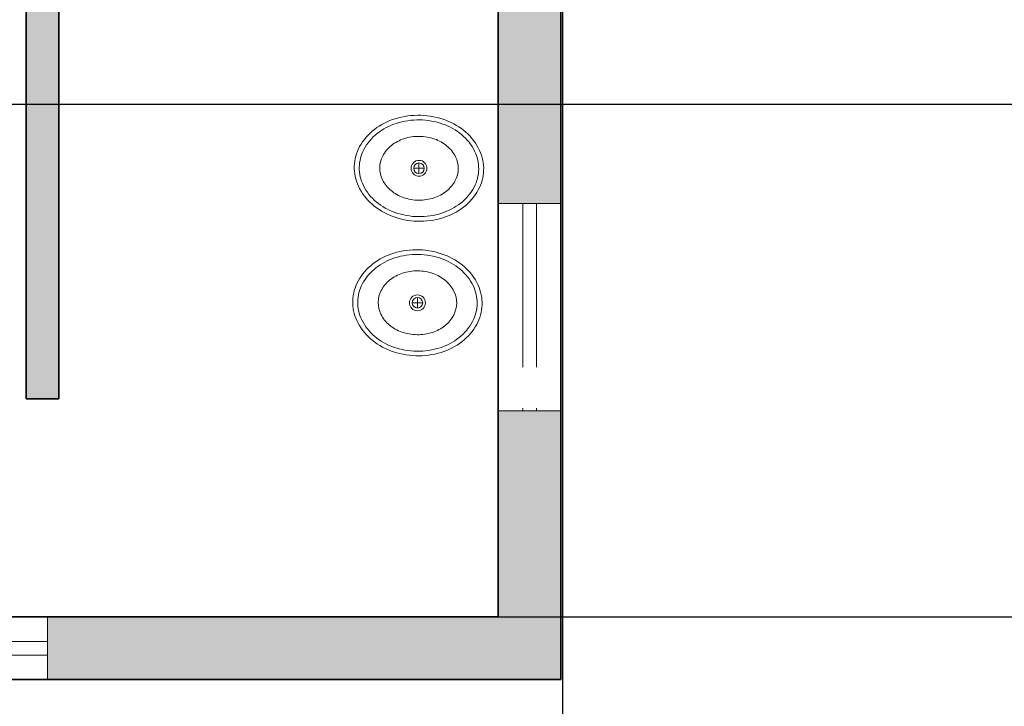
# Model space of a CAD drawing. Units: metres. Extents: x 4298.5 to 4325.2, y 2075 to 2095.8.
# Tile 27 of 35: x 4318.3 to 4321.9, y 2079.7 to 2082.2. Entities that reach past the tile are written whole.
import ezdxf

# ---------------------------------------------------------------- set-up
doc = ezdxf.new("R2010")
doc.units = ezdxf.units.M
doc.linetypes.add('ACAD_ISO02W100', pattern=[15, 12, -3])
for name, color, linetype, lineweight in [('A-ANNO-DIMS', 2, 'Continuous', 18), ('A-FLOR-FIXT', 15, 'Continuous', 18), ('A-GLAZ', 4, 'Continuous', 18), ('A-GLAZ-OVHD', 4, 'ACAD_ISO02W100', 13), ('A-WALL', 7, 'Continuous', 35), ('A-WALL-PATT', 252, 'Continuous', 13)]:
    doc.layers.add(name, color=color, linetype=linetype, lineweight=lineweight)
doc.styles.get("Standard").update_dxf_attribs({"font": 'arial.ttf'})
doc.dimstyles.get("Standard").update_dxf_attribs({"dimtxt": 0.18, "dimasz": 0.18, "dimexe": 0.18, "dimexo": 0.0625, "dimgap": 0.09, "dimtad": 0, "dimtih": 1, "dimtoh": 1, "dimdec": 4, "dimzin": 0, "dimdsep": 46, "dimtxsty": 'Standard', "dimcen": 0.09, "dimadec": 0, "dimazin": 0, "dimtfac": 1, "dimtdec": 4, "dimtofl": 0, "dimtmove": 0, "dimatfit": 3, "dimfxl": 1, "dimtolj": 1, "dimtzin": 0, "dimarcsym": 0})

# ---------------------------------------------------------------- blocks, each defined once
blk = doc.blocks.new('Sink - Oval top')
for p, q in [((-1, 0), (1, 0)), ((0, 1), (0, -1))]:
    blk.add_line(p, q)
for points in [[(-12.23, 0.39, 0.117634), (-11.46, -3.36, 0.104469), (-8.88, -6.8, 0.090016), (-5.08, -9.07, 0.08192), (-0.32, -10.02, 0.08192), (4.49, -9.38, 0.090016), (8.42, -7.36, 0.104469), (11.22, -4.09, 0.117634), (12.23, -0.39, 0.117634), (11.46, 3.36, 0.104469), (8.88, 6.8, 0.090016), (5.08, 9.07, 0.08192), (0.32, 10.02, 0.08192), (-4.49, 9.38, 0.090016), (-8.42, 7.36, 0.104469), (-11.22, 4.09, 0.117634)], [(-11.29, 0.16, 0.118622), (-10.52, -3.25, 0.104678), (-8.07, -6.36, 0.089562), (-4.54, -8.37, 0.081185), (-0.13, -9.15, 0.081185), (4.3, -8.49, 0.089562), (7.89, -6.58, 0.104678), (10.42, -3.55, 0.118622), (11.29, -0.16, 0.118622), (10.52, 3.25, 0.104678), (8.07, 6.36, 0.089562), (4.54, 8.37, 0.081185), (0.13, 9.15, 0.081185), (-4.3, 8.49, 0.089562), (-7.89, 6.58, 0.104678), (-10.42, 3.55, 0.118622)], [(-7.42, 0.08, 0.118283), (-6.91, -2.17, 0.104607), (-5.29, -4.21, 0.089718), (-2.97, -5.53, 0.081436), (-0.07, -6.04, 0.081436), (2.84, -5.59, 0.089718), (5.2, -4.33, 0.104607), (6.86, -2.32, 0.118283), (7.42, -0.08, 0.118283), (6.91, 2.17, 0.104607), (5.29, 4.21, 0.089718), (2.97, 5.53, 0.081436), (0.07, 6.04, 0.081436), (-2.84, 5.59, 0.089718), (-5.2, 4.33, 0.104607), (-6.86, 2.32, 0.118283)]]:
    blk.add_lwpolyline(points, format="xyb", close=True)
for radius in [1.5, 1]:
    blk.add_circle((0, 0), radius)
blk = doc.blocks.new('WIN-1000-GLASS')
for p, q in [((1, 0.05), (0, 0.05)), ((1, 0), (0, 0))]:
    blk.add_line(p, q)
blk = doc.blocks.new('WIN-760-GLASS-HIGH')
at = {"ltscale": 0.05}
for p, q in [((0, 0.76), (0, 0)), ((0.05, 0.76), (0.05, 0))]:
    blk.add_line(p, q, dxfattribs=at)
blk = doc.blocks.new('*D47')
at = {"layer": 'A-ANNO-DIMS', "color": 0, "lineweight": -2, "transparency": 16777216}
for p, q in [((4300.4306, 2084.4956), (4300.4306, 2074.9896)), ((4322.8106, 2084.4956), (4322.8106, 2074.9896)), ((4300.6106, 2075.1696), (4311.2252, 2075.1696)), ((4322.6306, 2075.1696), (4312.016, 2075.1696))]:
    blk.add_line(p, q, dxfattribs=at)
at = {"layer": 'A-ANNO-DIMS', "color": 0, "transparency": 16777216}
for points in [[(4300.6106, 2075.1996), (4300.6106, 2075.1396), (4300.4306, 2075.1696)], [(4322.6306, 2075.1996), (4322.6306, 2075.1396), (4322.8106, 2075.1696)]]:
    blk.add_solid(points, dxfattribs=at)
at = {"layer": 'Defpoints', "color": 0, "transparency": 16777216}
for p in [(4300.4306, 2084.5581), (4322.8106, 2084.5581), (4322.8106, 2075.1696)]:
    blk.add_point(p, dxfattribs=at)
at = {"layer": 'A-ANNO-DIMS', "color": 0, "transparency": 16777216, "insert": (4311.6206, 2075.1696), "char_height": 0.18, "attachment_point": 5}
blk.add_mtext('\\A1;22.38', dxfattribs=at)
blk = doc.blocks.new('*D48')
at = {"layer": 'A-ANNO-DIMS', "color": 0, "lineweight": -2, "transparency": 16777216}
for p, q in [((4310.1831, 2094.4781), (4324.7671, 2094.4781)), ((4324.5871, 2094.2981), (4324.5871, 2085.585)), ((4324.5871, 2076.5081), (4324.5871, 2085.2212)), ((4316.8731, 2076.3281), (4324.7671, 2076.3281))]:
    blk.add_line(p, q, dxfattribs=at)
at = {"layer": 'A-ANNO-DIMS', "color": 0, "transparency": 16777216}
for points in [[(4324.5571, 2094.2981), (4324.6171, 2094.2981), (4324.5871, 2094.4781)], [(4324.5571, 2076.5081), (4324.6171, 2076.5081), (4324.5871, 2076.3281)]]:
    blk.add_solid(points, dxfattribs=at)
at = {"layer": 'Defpoints', "color": 0, "transparency": 16777216}
for p in [(4310.1206, 2094.4781), (4316.8106, 2076.3281), (4324.5871, 2076.3281)]:
    blk.add_point(p, dxfattribs=at)
at = {"layer": 'A-ANNO-DIMS', "color": 0, "transparency": 16777216, "insert": (4324.5871, 2085.4031), "char_height": 0.18, "attachment_point": 5}
blk.add_mtext('\\A1;18.15', dxfattribs=at)
blk = doc.blocks.new('*D55')
at = {"layer": 'A-ANNO-DIMS', "color": 0, "lineweight": -2, "transparency": 16777216}
for p, q in [((4320.3167, 2084.4996), (4320.3167, 2074.9896)), ((4322.8106, 2084.4956), (4322.8106, 2074.9896)), ((4320.4967, 2075.1696), (4321.1688, 2075.1696)), ((4322.6306, 2075.1696), (4321.9585, 2075.1696))]:
    blk.add_line(p, q, dxfattribs=at)
at = {"layer": 'A-ANNO-DIMS', "color": 0, "transparency": 16777216}
for points in [[(4320.4967, 2075.1996), (4320.4967, 2075.1396), (4320.3167, 2075.1696)], [(4322.6306, 2075.1996), (4322.6306, 2075.1396), (4322.8106, 2075.1696)]]:
    blk.add_solid(points, dxfattribs=at)
at = {"layer": 'Defpoints', "color": 0, "transparency": 16777216}
for p in [(4320.3167, 2084.5621), (4322.8106, 2084.5581), (4322.8106, 2075.1696)]:
    blk.add_point(p, dxfattribs=at)
at = {"layer": 'A-ANNO-DIMS', "color": 0, "transparency": 16777216, "insert": (4321.5636, 2075.1696), "char_height": 0.18, "attachment_point": 5}
blk.add_mtext('\\A1;2.494', dxfattribs=at)
blk = doc.blocks.new('*D60')
at = {"layer": 'A-ANNO-DIMS', "color": 0, "lineweight": -2, "transparency": 16777216}
for p, q in [((4305.9531, 2081.9381), (4324.7671, 2081.9381)), ((4324.5871, 2081.7581), (4324.5871, 2081.18)), ((4324.5871, 2080.2381), (4324.5871, 2080.8162)), ((4305.9531, 2080.0581), (4324.7671, 2080.0581))]:
    blk.add_line(p, q, dxfattribs=at)
at = {"layer": 'A-ANNO-DIMS', "color": 0, "transparency": 16777216}
for points in [[(4324.5571, 2081.7581), (4324.6171, 2081.7581), (4324.5871, 2081.9381)], [(4324.5571, 2080.2381), (4324.6171, 2080.2381), (4324.5871, 2080.0581)]]:
    blk.add_solid(points, dxfattribs=at)
at = {"layer": 'Defpoints', "color": 0, "transparency": 16777216}
for p in [(4305.8906, 2081.9381), (4324.5871, 2081.9381), (4305.8906, 2080.0581)]:
    blk.add_point(p, dxfattribs=at)
at = {"layer": 'A-ANNO-DIMS', "color": 0, "transparency": 16777216, "insert": (4324.5871, 2080.9981), "char_height": 0.18, "attachment_point": 5}
blk.add_mtext('\\A1;1.88', dxfattribs=at)
blk = doc.blocks.new('*D79')
at = {"layer": 'A-ANNO-DIMS', "color": 0, "lineweight": -2, "transparency": 16777216}
for p, q in [((4313.4743, 2079.7393), (4313.4743, 2079.9193)), ((4313.3843, 2079.8293), (4313.5643, 2079.8293)), ((4320.4622, 2076.981), (4318.0084, 2077.9812)), ((4320.6422, 2076.981), (4320.4622, 2076.981))]:
    blk.add_line(p, q, dxfattribs=at)
at = {"layer": 'A-ANNO-DIMS', "color": 0, "transparency": 16777216}
blk.add_solid([(4318.0197, 2078.009), (4317.9971, 2077.9534), (4317.8417, 2078.0491)], dxfattribs=at)
at = {"layer": 'Defpoints', "color": 0, "transparency": 16777216}
for p in [(4313.4743, 2079.8293), (4317.8417, 2078.0491)]:
    blk.add_point(p, dxfattribs=at)
at = {"layer": 'A-ANNO-DIMS', "color": 0, "transparency": 16777216, "insert": (4321.3169, 2076.981), "char_height": 0.18, "attachment_point": 5}
blk.add_mtext('\\A1;2X R4.716', dxfattribs=at)

msp = doc.modelspace()

# ---------------------------------------------------------------- hatches: boundary and pattern name
at = {"layer": 'A-WALL-PATT'}
h = msp.add_hatch(color=256, dxfattribs=at)
h.dxf.hatch_style = 1
h.paths.add_polyline_path([(4308.7606, 2094.4781), (4308.1606, 2094.4781), (4307.4606, 2094.4781), (4307.4606, 2094.2481), (4308.2706, 2094.2481), (4308.2706, 2094.1281), (4308.3906, 2094.1281), (4308.3906, 2094.2481), (4308.7606, 2094.2481)])
h.paths.add_polyline_path([(4310.1206, 2094.4781), (4309.5206, 2094.4781), (4309.5206, 2094.2481), (4309.8906, 2094.2481), (4309.8906, 2092.2481), (4308.3906, 2092.2481), (4308.3906, 2093.4281), (4308.2706, 2093.4281), (4308.2706, 2092.0181), (4309.8906, 2092.0181), (4309.8906, 2087.0181), (4309.7706, 2087.0181), (4309.7706, 2086.7881), (4309.8906, 2086.7881), (4311.9406, 2086.7881), (4311.9406, 2087.0181), (4310.1206, 2087.0181), (4310.1206, 2089.0181), (4310.2406, 2089.0181), (4310.2406, 2089.1381), (4310.1206, 2089.1381), (4310.1206, 2092.0181), (4310.3078, 2092.0181), (4310.3078, 2092.2481), (4310.1206, 2092.2481)])
h.paths.add_polyline_path([(4311.7406, 2092.2481), (4311.0678, 2092.2481), (4311.0678, 2092.0181), (4311.7406, 2092.0181)], flags=17)
h.paths.add_polyline_path([(4313.1733, 2092.2481), (4312.5006, 2092.2481), (4312.5006, 2092.0181), (4313.1733, 2092.0181)])
h.paths.add_polyline_path([(4314.5378, 2092.2481), (4314.1206, 2092.2481), (4313.9333, 2092.2481), (4313.9333, 2092.0181), (4314.1206, 2092.0181), (4314.1206, 2087.0181), (4314.0006, 2087.0181), (4314.0006, 2086.7881), (4314.1206, 2086.7881), (4315.5718, 2086.7881), (4315.5718, 2087.0181), (4314.3506, 2087.0181), (4314.3506, 2092.0181), (4314.5378, 2092.0181)])
h.paths.add_polyline_path([(4315.9706, 2092.2481), (4315.2978, 2092.2481), (4315.2978, 2092.0181), (4315.9706, 2092.0181)])
h.paths.add_polyline_path([(4317.4033, 2092.2481), (4316.7306, 2092.2481), (4316.7306, 2092.0181), (4317.4033, 2092.0181)])
h.paths.add_polyline_path([(4318.9506, 2092.2481), (4318.3506, 2092.2481), (4318.1633, 2092.2481), (4318.1633, 2092.0181), (4318.3506, 2092.0181), (4318.3506, 2091.8981), (4318.5806, 2091.8981), (4318.5806, 2092.0181), (4318.9506, 2092.0181)])
h.paths.add_polyline_path([(4321.0106, 2092.2481), (4319.7106, 2092.2481), (4319.7106, 2092.0181), (4320.0806, 2092.0181), (4320.0806, 2090.0181), (4318.5806, 2090.0181), (4318.5806, 2091.1981), (4318.3506, 2091.1981), (4318.3506, 2090.0181), (4318.3506, 2087.0181), (4318.2306, 2087.0181), (4318.2306, 2086.7881), (4318.3506, 2086.7881), (4318.3506, 2086.3081), (4318.5806, 2086.3081), (4318.5806, 2089.7881), (4321.7806, 2089.7881), (4321.7806, 2090.0181), (4320.2006, 2090.0181), (4320.2006, 2092.0181), (4321.0106, 2092.0181)])
h.paths.add_polyline_path([(4322.8106, 2092.2481), (4321.7706, 2092.2481), (4321.7706, 2092.0181), (4322.5806, 2092.0181), (4322.5806, 2091.2831), (4322.8106, 2091.2831)])
h.paths.add_polyline_path([(4322.8106, 2090.5231), (4322.5806, 2090.5231), (4322.5806, 2089.7881), (4322.5806, 2089.5254), (4322.8106, 2089.5254), (4322.8106, 2090.0181)])
h.paths.add_polyline_path([(4322.8106, 2088.7654), (4322.5806, 2088.7654), (4322.5806, 2087.6681), (4322.8106, 2087.6681)])
h.paths.add_polyline_path([(4322.8106, 2086.9081), (4322.5806, 2086.9081), (4322.5806, 2085.8107), (4322.8106, 2085.8107)])
h.paths.add_polyline_path([(4322.8106, 2085.0507), (4322.5806, 2085.0507), (4322.5806, 2084.7881), (4318.5806, 2084.7881), (4318.5806, 2085.0581), (4318.5806, 2085.4081), (4318.3506, 2085.4081), (4318.3506, 2084.5581), (4318.3506, 2080.8581), (4318.4706, 2080.8581), (4318.4706, 2082.3281), (4319.2606, 2082.3281), (4319.2606, 2082.5581), (4318.5806, 2082.5581), (4318.5806, 2084.5581), (4320.0806, 2084.5581), (4320.0806, 2083.9381), (4320.3106, 2083.9381), (4320.3106, 2084.5581), (4322.8106, 2084.5581)])
h.paths.add_polyline_path([(4320.3106, 2083.1781), (4320.0806, 2083.1781), (4320.0806, 2082.5581), (4319.9606, 2082.5581), (4319.9606, 2082.3281), (4320.0806, 2082.3281), (4320.0806, 2081.5731), (4320.3106, 2081.5731)], flags=17)
h.paths.add_polyline_path([(4320.3106, 2080.8131), (4320.0806, 2080.8131), (4320.0806, 2080.0581), (4318.4286, 2080.0581), (4318.4286, 2079.8281), (4320.3106, 2079.8281)])
h.paths.add_polyline_path([(4317.3506, 2085.2881), (4316.5718, 2085.2881), (4316.5718, 2085.0581), (4317.3506, 2085.0581)])
h.paths.add_polyline_path([(4315.5718, 2085.2881), (4314.8434, 2085.2881), (4314.8434, 2085.0581), (4315.5718, 2085.0581)])
h.paths.add_polyline_path([(4313.8434, 2085.2881), (4312.9406, 2085.2881), (4312.9406, 2085.0581), (4313.8434, 2085.0581)])
h.paths.add_polyline_path([(4311.9406, 2085.2881), (4311.4406, 2085.2881), (4311.4406, 2085.0581), (4311.9406, 2085.0581)])
h.paths.add_polyline_path([(4317.3306, 2087.0181), (4316.5718, 2087.0181), (4316.5718, 2086.7881), (4317.3306, 2086.7881)])
h.paths.add_polyline_path([(4313.1006, 2089.1381), (4311.1406, 2089.1381), (4311.1406, 2089.0181), (4312.9806, 2089.0181), (4312.9806, 2087.0181), (4312.9406, 2087.0181), (4312.9406, 2086.7881), (4313.1006, 2086.7881), (4313.1006, 2087.0181)])
h.paths.add_polyline_path([(4307.5515, 2087.0181), (4305.8906, 2087.0181), (4305.8906, 2092.2481), (4305.8906, 2094.2481), (4306.7006, 2094.2481), (4306.7006, 2094.4781), (4305.6606, 2094.4781), (4305.6606, 2092.2481), (4305.2906, 2092.2481), (4305.2906, 2092.0181), (4305.6606, 2092.0181), (4305.6606, 2090.0181), (4304.1606, 2090.0181), (4304.1606, 2091.1981), (4304.0406, 2091.1981), (4304.0406, 2089.9081), (4301.5606, 2089.9081), (4301.5606, 2089.7881), (4304.0406, 2089.7881), (4305.6606, 2089.7881), (4305.6606, 2086.6381), (4305.8906, 2086.6381), (4305.8906, 2086.7881), (4307.5515, 2086.7881)])
h.paths.add_polyline_path([(4307.5515, 2085.2881), (4305.8906, 2085.2881), (4305.8906, 2085.4381), (4305.6606, 2085.4381), (4305.6606, 2084.7881), (4305.2906, 2084.7881), (4305.2906, 2084.5581), (4305.6606, 2084.5581), (4305.6606, 2084.02), (4305.8906, 2084.02), (4305.8906, 2084.5581), (4305.8906, 2085.0581), (4307.5515, 2085.0581)])
h.paths.add_polyline_path([(4310.2406, 2085.2881), (4308.5515, 2085.2881), (4308.5515, 2085.0581), (4310.2406, 2085.0581)])
h.paths.add_polyline_path([(4317.4286, 2080.0581), (4316.5718, 2080.0581), (4316.5718, 2079.8281), (4317.4286, 2079.8281)])
h.paths.add_polyline_path([(4315.5718, 2080.0581), (4314.8434, 2080.0581), (4314.8434, 2079.8281), (4315.5718, 2079.8281)])
h.paths.add_polyline_path([(4313.8434, 2080.0581), (4312.9406, 2080.0581), (4312.9406, 2079.8281), (4313.8434, 2079.8281)])
h.paths.add_polyline_path([(4311.9406, 2080.0581), (4311.4406, 2080.0581), (4311.4406, 2079.8281), (4311.9406, 2079.8281)])
h.paths.add_polyline_path([(4310.2406, 2080.0581), (4310.1206, 2080.0581), (4310.1206, 2084.0381), (4309.8906, 2084.0381), (4309.8906, 2080.0581), (4309.1606, 2080.0581), (4309.1606, 2079.8281), (4310.2406, 2079.8281)])
h.paths.add_polyline_path([(4308.1606, 2080.0581), (4307.5106, 2080.0581), (4307.5106, 2080.1781), (4307.3906, 2080.1781), (4307.3906, 2080.0581), (4305.8906, 2080.0581), (4305.8906, 2080.567), (4305.6606, 2080.567), (4305.6606, 2079.8281), (4308.1606, 2079.8281)])
h.paths.add_polyline_path([(4307.5106, 2081.9381), (4309.0906, 2081.9381), (4309.0906, 2082.0581), (4305.8906, 2082.0581), (4305.8906, 2083.26), (4305.6606, 2083.26), (4305.6606, 2081.327), (4305.8906, 2081.327), (4305.8906, 2081.9381), (4307.3906, 2081.9381), (4307.3906, 2080.8781), (4307.5106, 2080.8781)])
h.paths.add_polyline_path([(4304.5306, 2084.7881), (4302.7306, 2084.7881), (4302.7306, 2084.5581), (4304.5306, 2084.5581)])
h.paths.add_polyline_path([(4301.9706, 2084.7881), (4300.6606, 2084.7881), (4300.6606, 2085.0249), (4300.4306, 2085.0249), (4300.4306, 2084.5581), (4301.9706, 2084.5581)])
h.paths.add_polyline_path([(4300.6606, 2086.8843), (4300.4306, 2086.8843), (4300.4306, 2085.7849), (4300.6606, 2085.7849)])
h.paths.add_polyline_path([(4300.6606, 2089.1618), (4300.4306, 2089.1618), (4300.4306, 2087.6443), (4300.6606, 2087.6443)])
h.paths.add_polyline_path([(4300.6606, 2091.0212), (4300.4306, 2091.0212), (4300.4306, 2089.9218), (4300.6606, 2089.9218)])
h.paths.add_polyline_path([(4300.6606, 2092.0181), (4301.9706, 2092.0181), (4301.9706, 2092.2481), (4300.4306, 2092.2481), (4300.4306, 2091.7812), (4300.6606, 2091.7812)])
h.paths.add_polyline_path([(4304.5306, 2092.2481), (4302.7306, 2092.2481), (4302.7306, 2092.0181), (4304.0406, 2092.0181), (4304.0406, 2091.8981), (4304.1606, 2091.8981), (4304.1606, 2092.0181), (4304.5306, 2092.0181)], flags=17)

# ---------------------------------------------------------------- linework, layer by layer
at = {"layer": 'A-GLAZ'}
for p, q in [((4320.0806, 2081.5731), (4320.3106, 2081.5731)), ((4320.0806, 2080.8131), (4320.3106, 2080.8131)), ((4318.4286, 2079.8281), (4318.4286, 2080.0581))]:
    msp.add_line(p, q, dxfattribs=at)
at = {"layer": 'A-WALL'}
for p, q in [((4318.3506, 2085.0581), (4318.3506, 2080.8581)), ((4320.3106, 2084.5581), (4320.3106, 2079.8281)), ((4318.4706, 2082.3281), (4318.4706, 2080.8581)), ((4320.0806, 2082.3281), (4320.0806, 2080.0581)), ((4318.3506, 2080.8581), (4318.4706, 2080.8581)), ((4318.3506, 2080.0581), (4311.4156, 2080.0581)), ((4320.0806, 2080.0581), (4318.3506, 2080.0581)), ((4320.3106, 2079.8281), (4311.4406, 2079.8281))]:
    msp.add_line(p, q, dxfattribs=at)

# ---------------------------------------------------------------- block references
at = {"layer": 'A-FLOR-FIXT', "xscale": 0.0193818050953029, "yscale": 0.0193818050953029, "zscale": 0.0193818050953029}
for p in [(4319.7905, 2081.7027), (4319.7848, 2081.2096)]:
    msp.add_blockref('Sink - Oval top', p, dxfattribs=at)
at = {"layer": 'A-GLAZ'}
msp.add_blockref('WIN-1000-GLASS', (4317.4286, 2079.9181), dxfattribs=at)
at = {"layer": 'A-GLAZ-OVHD'}
msp.add_blockref('WIN-760-GLASS-HIGH', (4320.1706, 2080.8131), dxfattribs=at)

# ---------------------------------------------------------------- dimensions: what is measured, and where the dimension line sits
at = {"layer": 'A-ANNO-DIMS'}
for base, p1, p2, picture, middle in [((4324.5871, 2076.3281), (4310.1206, 2094.4781), (4316.8106, 2076.3281), '*D48', (4324.5871, 2085.4031)), ((4324.5871, 2081.9381), (4305.8906, 2080.0581), (4305.8906, 2081.9381), '*D60', (4324.5871, 2080.9981))]:
    dim = msp.add_linear_dim(base=base, p1=p1, p2=p2, angle=90, dimstyle='Standard', override={"dimdec": 2, "dimlfac": 1, "dimrnd": 0, "dimzin": 0, "dimdsep": 46, "dimlunit": 2}, dxfattribs=at)
    dim.commit()
    dim.dimension.update_dxf_attribs({"geometry": picture, "text_midpoint": middle})
for p1, override, picture, middle in [((4300.4306, 2084.5581), {"dimdec": 2, "dimlfac": 1, "dimrnd": 0, "dimzin": 0, "dimdsep": 46, "dimlunit": 2}, '*D47', (4311.6206, 2075.1696)), ((4320.3167, 2084.5621), {"dimdec": 3, "dimlfac": 1, "dimrnd": 0, "dimzin": 0, "dimdsep": 46, "dimlunit": 2}, '*D55', (4321.5636, 2075.1696))]:
    dim = msp.add_linear_dim(base=(4322.8106, 2075.1696), p1=p1, p2=(4322.8106, 2084.5581), dimstyle='Standard', override=override, dxfattribs=at)
    dim.commit()
    dim.dimension.update_dxf_attribs({"geometry": picture, "text_midpoint": middle})
dim = msp.add_radius_dim(center=(4313.4743, 2079.8293), mpoint=(4317.8417, 2078.0491), text='2X <>', dimstyle='Standard', override={"dimdec": 3, "dimlfac": 1, "dimrnd": 0, "dimzin": 0, "dimdsep": 46, "dimlunit": 2}, dxfattribs=at)
dim.commit()
dim.dimension.update_dxf_attribs({"geometry": '*D79', "text_midpoint": (4321.3169, 2076.981), "dimtype": 164})

doc.saveas('drawing.dxf')
